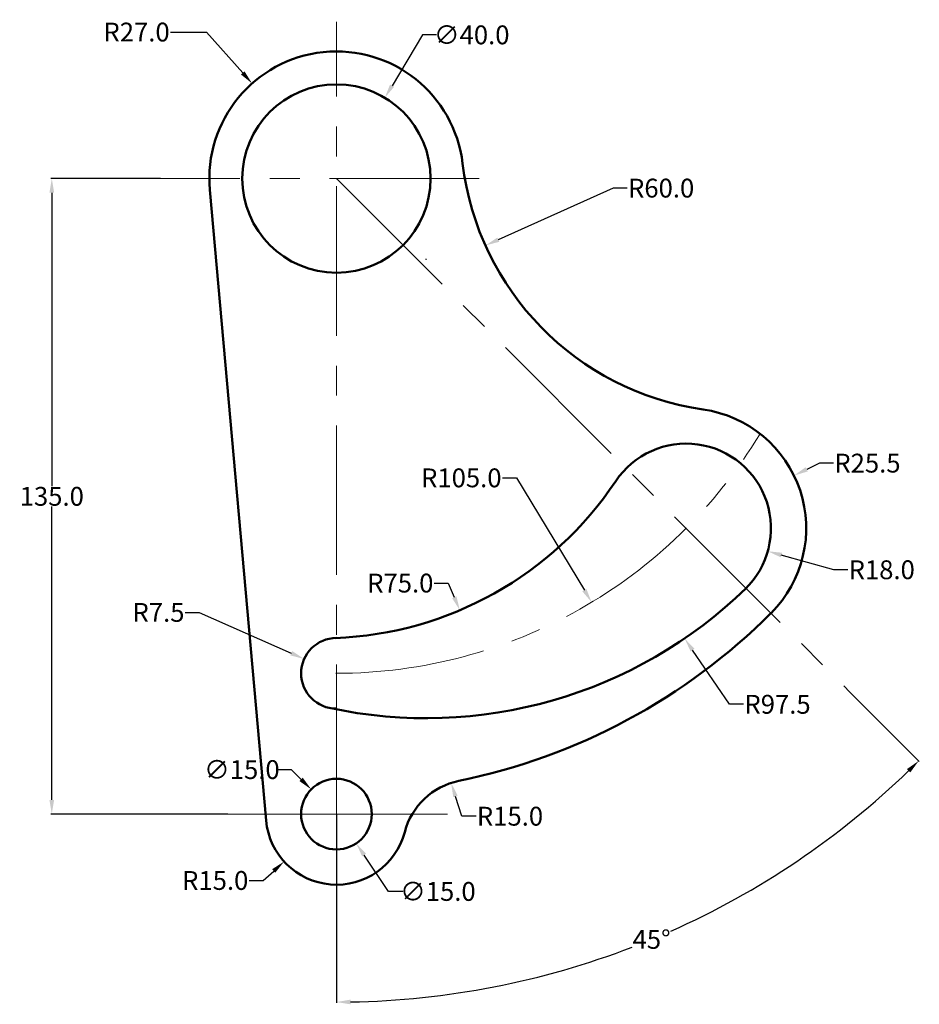
# Model space of a CAD drawing. Units: inches. Extents: x 482 to 673, y 355 to 564.
import ezdxf

# ---------------------------------------------------------------- set-up
doc = ezdxf.new("R2010")
doc.units = ezdxf.units.IN
doc.header["$MEASUREMENT"] = 0
doc.linetypes.add('CENTER', pattern=[50.8, 31.75, -6.35, 6.35, -6.35])
for name, color, linetype, lineweight in [('M-CNTR', 4, 'CENTER', 18), ('M-DIMS', 2, 'Continuous', 25), ('M-OUTL', 7, 'Continuous', 50)]:
    doc.layers.add(name, color=color, linetype=linetype, lineweight=lineweight)
doc.styles.get("Standard").update_dxf_attribs({"font": 'arial.ttf'})
doc.dimstyles.get("Standard").update_dxf_attribs({"dimtxt": 4, "dimasz": 3, "dimexe": 0.18, "dimexo": 0.0625, "dimgap": 0.09, "dimtad": 0, "dimtih": 1, "dimtoh": 1, "dimdec": 1, "dimzin": 0, "dimdsep": 46, "dimtxsty": 'Standard', "dimcen": 0.09, "dimadec": 0, "dimazin": 0, "dimtfac": 1, "dimtdec": 1, "dimtofl": 0, "dimtmove": 0, "dimatfit": 3, "dimfxl": 1, "dimtolj": 1, "dimtzin": 0, "dimarcsym": 0})

# ---------------------------------------------------------------- blocks, each defined once
blk = doc.blocks.new('*D1')
at = {"layer": 'Defpoints', "color": 0, "transparency": 16777216}
for p in [(531.06, 550.32), (548.98, 530.12)]:
    blk.add_point(p, dxfattribs=at)
at = {"layer": 'M-DIMS', "color": 0, "lineweight": -2, "transparency": 16777216}
for p, q in [((513.71, 561.24), (521.37, 561.24)), ((521.37, 561.24), (529.07, 552.56)), ((548.89, 530.12), (549.07, 530.12)), ((548.98, 530.03), (548.98, 530.21))]:
    blk.add_line(p, q, dxfattribs=at)
at = {"layer": 'M-DIMS', "color": 0, "transparency": 16777216}
blk.add_solid([(529.45, 552.89), (528.7, 552.23), (531.06, 550.32)], dxfattribs=at)
at = {"layer": 'M-DIMS', "color": 0, "transparency": 16777216, "insert": (506.52, 561.24), "char_height": 4, "attachment_point": 5}
blk.add_mtext('\\A1;R27.0', dxfattribs=at)
blk = doc.blocks.new('*D2')
at = {"layer": 'Defpoints', "color": 0, "transparency": 16777216}
for p in [(559.26, 547.28), (538.71, 512.96)]:
    blk.add_point(p, dxfattribs=at)
at = {"layer": 'M-DIMS', "color": 0, "lineweight": -2, "transparency": 16777216}
for p, q in [((567.26, 560.64), (560.8, 549.85)), ((570.26, 560.64), (567.26, 560.64)), ((548.89, 530.12), (549.07, 530.12)), ((548.98, 530.03), (548.98, 530.21))]:
    blk.add_line(p, q, dxfattribs=at)
at = {"layer": 'M-DIMS', "color": 0, "transparency": 16777216}
blk.add_solid([(560.37, 550.11), (561.23, 549.6), (559.26, 547.28)], dxfattribs=at)
at = {"layer": 'M-DIMS', "color": 0, "transparency": 16777216, "insert": (577.72, 560.64), "char_height": 4, "attachment_point": 5}
blk.add_mtext('\\A1;∅40.0', dxfattribs=at)
blk = doc.blocks.new('*D3')
at = {"layer": 'Defpoints', "color": 0, "transparency": 16777216}
for p in [(635.37, 540.47), (580.63, 515.91)]:
    blk.add_point(p, dxfattribs=at)
at = {"layer": 'M-DIMS', "color": 0, "lineweight": -2, "transparency": 16777216}
for p, q in [((607.77, 528.09), (583.36, 517.13)), ((610.77, 528.09), (607.77, 528.09))]:
    blk.add_line(p, q, dxfattribs=at)
at = {"layer": 'M-DIMS', "color": 0, "transparency": 16777216}
blk.add_solid([(583.16, 517.59), (583.57, 516.68), (580.63, 515.91)], dxfattribs=at)
at = {"layer": 'M-DIMS', "color": 0, "transparency": 16777216, "insert": (617.96, 528.09), "char_height": 4, "attachment_point": 5}
blk.add_mtext('\\A1;R60.0', dxfattribs=at)
blk = doc.blocks.new('*D4')
at = {"layer": 'Defpoints', "color": 0, "transparency": 16777216}
for p in [(646.18, 467.03), (623.28, 455.83)]:
    blk.add_point(p, dxfattribs=at)
at = {"layer": 'M-DIMS', "color": 0, "lineweight": -2, "transparency": 16777216}
for p, q in [((651.57, 469.67), (648.88, 468.35)), ((654.57, 469.67), (651.57, 469.67)), ((623.19, 455.83), (623.37, 455.83)), ((623.28, 455.74), (623.28, 455.92))]:
    blk.add_line(p, q, dxfattribs=at)
at = {"layer": 'M-DIMS', "color": 0, "transparency": 16777216}
blk.add_solid([(648.66, 468.8), (649.1, 467.9), (646.18, 467.03)], dxfattribs=at)
at = {"layer": 'M-DIMS', "color": 0, "transparency": 16777216, "insert": (661.79, 469.67), "char_height": 4, "attachment_point": 5}
blk.add_mtext('\\A1;R25.5', dxfattribs=at)
blk = doc.blocks.new('*D5')
at = {"layer": 'Defpoints', "color": 0, "transparency": 16777216}
for p in [(623.28, 455.83), (640.6, 450.96)]:
    blk.add_point(p, dxfattribs=at)
at = {"layer": 'M-DIMS', "color": 0, "lineweight": -2, "transparency": 16777216}
for p, q in [((623.19, 455.83), (623.37, 455.83)), ((623.28, 455.74), (623.28, 455.92)), ((654.63, 447.02), (643.49, 450.15)), ((657.63, 447.02), (654.63, 447.02))]:
    blk.add_line(p, q, dxfattribs=at)
at = {"layer": 'M-DIMS', "color": 0, "transparency": 16777216}
blk.add_solid([(643.63, 450.63), (643.36, 449.67), (640.6, 450.96)], dxfattribs=at)
at = {"layer": 'M-DIMS', "color": 0, "transparency": 16777216, "insert": (664.82, 447.02), "char_height": 4, "attachment_point": 5}
blk.add_mtext('\\A1;R18.0', dxfattribs=at)
blk = doc.blocks.new('*D6')
at = {"layer": 'Defpoints', "color": 0, "transparency": 16777216}
for p in [(568.03, 512.99), (622.94, 432.43)]:
    blk.add_point(p, dxfattribs=at)
at = {"layer": 'M-DIMS', "color": 0, "lineweight": -2, "transparency": 16777216}
for p, q in [((567.94, 512.99), (568.12, 512.99)), ((568.03, 512.9), (568.03, 513.08)), ((632.48, 418.44), (624.63, 429.95)), ((635.48, 418.44), (632.48, 418.44))]:
    blk.add_line(p, q, dxfattribs=at)
at = {"layer": 'M-DIMS', "color": 0, "transparency": 16777216}
blk.add_solid([(625.04, 430.23), (624.22, 429.67), (622.94, 432.43)], dxfattribs=at)
at = {"layer": 'M-DIMS', "color": 0, "transparency": 16777216, "insert": (642.69, 418.44), "char_height": 4, "attachment_point": 5}
blk.add_mtext('\\A1;R97.5', dxfattribs=at)
blk = doc.blocks.new('*D7')
at = {"layer": 'Defpoints', "color": 0, "transparency": 16777216}
for p in [(548.98, 530.03), (603.2, 440.11)]:
    blk.add_point(p, dxfattribs=at)
at = {"layer": 'M-DIMS', "color": 0, "lineweight": -2, "transparency": 16777216}
for p, q in [((584.26, 466.54), (587.26, 466.54)), ((587.26, 466.54), (601.65, 442.68))]:
    blk.add_line(p, q, dxfattribs=at)
at = {"layer": 'M-DIMS', "color": 0, "transparency": 16777216}
blk.add_solid([(602.08, 442.94), (601.22, 442.42), (603.2, 440.11)], dxfattribs=at)
at = {"layer": 'M-DIMS', "color": 0, "transparency": 16777216, "insert": (575.51, 466.54), "char_height": 4, "attachment_point": 5}
blk.add_mtext('\\A1;R105.0', dxfattribs=at)
blk = doc.blocks.new('*D8')
at = {"layer": 'Defpoints', "color": 0, "transparency": 16777216}
for p in [(545.93, 507.47), (575.19, 438.42)]:
    blk.add_point(p, dxfattribs=at)
at = {"layer": 'M-DIMS', "color": 0, "lineweight": -2, "transparency": 16777216}
for p, q in [((569.74, 444.19), (572.74, 444.19)), ((572.74, 444.19), (574.02, 441.18))]:
    blk.add_line(p, q, dxfattribs=at)
at = {"layer": 'M-DIMS', "color": 0, "transparency": 16777216}
blk.add_solid([(574.48, 441.37), (573.56, 440.98), (575.19, 438.42)], dxfattribs=at)
at = {"layer": 'M-DIMS', "color": 0, "transparency": 16777216, "insert": (562.55, 444.19), "char_height": 4, "attachment_point": 5}
blk.add_mtext('\\A1;R75.0', dxfattribs=at)
blk = doc.blocks.new('*D9')
at = {"layer": 'Defpoints', "color": 0, "transparency": 16777216}
for p in [(542.13, 428.07), (548.98, 425.03)]:
    blk.add_point(p, dxfattribs=at)
at = {"layer": 'M-DIMS', "color": 0, "lineweight": -2, "transparency": 16777216}
for p, q in [((516.84, 437.96), (519.84, 437.96)), ((519.84, 437.96), (539.39, 429.29)), ((548.89, 425.03), (549.07, 425.03)), ((548.98, 424.94), (548.98, 425.12))]:
    blk.add_line(p, q, dxfattribs=at)
at = {"layer": 'M-DIMS', "color": 0, "transparency": 16777216}
blk.add_solid([(539.59, 429.75), (539.18, 428.83), (542.13, 428.07)], dxfattribs=at)
at = {"layer": 'M-DIMS', "color": 0, "transparency": 16777216, "insert": (511.18, 437.96), "char_height": 4, "attachment_point": 5}
blk.add_mtext('\\A1;R7.5', dxfattribs=at)
blk = doc.blocks.new('*D10')
at = {"layer": 'Defpoints', "color": 0, "transparency": 16777216}
for p in [(548.98, 395.12), (537.87, 385.05)]:
    blk.add_point(p, dxfattribs=at)
at = {"layer": 'M-DIMS', "color": 0, "lineweight": -2, "transparency": 16777216}
for p, q in [((548.89, 395.12), (549.07, 395.12)), ((548.98, 395.03), (548.98, 395.21)), ((533.42, 381.02), (535.65, 383.03)), ((530.42, 381.02), (533.42, 381.02))]:
    blk.add_line(p, q, dxfattribs=at)
at = {"layer": 'M-DIMS', "color": 0, "transparency": 16777216}
blk.add_solid([(535.31, 383.4), (535.98, 382.66), (537.87, 385.05)], dxfattribs=at)
at = {"layer": 'M-DIMS', "color": 0, "transparency": 16777216, "insert": (523.23, 381.02), "char_height": 4, "attachment_point": 5}
blk.add_mtext('\\A1;R15.0', dxfattribs=at)
blk = doc.blocks.new('*D11')
at = {"layer": 'Defpoints', "color": 0, "transparency": 16777216}
for p in [(544.79, 401.34), (553.18, 388.9)]:
    blk.add_point(p, dxfattribs=at)
at = {"layer": 'M-DIMS', "color": 0, "lineweight": -2, "transparency": 16777216}
for p, q in [((548.89, 395.12), (549.07, 395.12)), ((548.98, 395.03), (548.98, 395.21)), ((560.07, 378.69), (554.86, 386.42)), ((563.07, 378.69), (560.07, 378.69))]:
    blk.add_line(p, q, dxfattribs=at)
at = {"layer": 'M-DIMS', "color": 0, "transparency": 16777216}
blk.add_solid([(555.27, 386.7), (554.44, 386.14), (553.18, 388.9)], dxfattribs=at)
at = {"layer": 'M-DIMS', "color": 0, "transparency": 16777216, "insert": (570.53, 378.69), "char_height": 4, "attachment_point": 5}
blk.add_mtext('\\A1;∅15.0', dxfattribs=at)
blk = doc.blocks.new('*D12')
at = {"layer": 'Defpoints', "color": 0, "transparency": 16777216}
for p in [(573.35, 401.74), (577.99, 387.48)]:
    blk.add_point(p, dxfattribs=at)
at = {"layer": 'M-DIMS', "color": 0, "lineweight": -2, "transparency": 16777216}
for p, q in [((575.65, 394.67), (574.28, 398.89)), ((578.65, 394.67), (575.65, 394.67))]:
    blk.add_line(p, q, dxfattribs=at)
at = {"layer": 'M-DIMS', "color": 0, "transparency": 16777216}
blk.add_solid([(574.75, 399.04), (573.8, 398.73), (573.35, 401.74)], dxfattribs=at)
at = {"layer": 'M-DIMS', "color": 0, "transparency": 16777216, "insert": (585.85, 394.67), "char_height": 4, "attachment_point": 5}
blk.add_mtext('\\A1;R15.0', dxfattribs=at)
blk = doc.blocks.new('*D13')
at = {"layer": 'Defpoints', "color": 0, "transparency": 16777216}
for p in [(548.98, 530.12), (548.98, 530.12), (657.39, 421.72), (548.98, 395.12), (594.26, 361.15)]:
    blk.add_point(p, dxfattribs=at)
at = {"layer": 'M-DIMS', "color": 0, "lineweight": -2, "transparency": 16777216}
for p, q in [((657.43, 421.67), (672.81, 406.3)), ((548.98, 395.06), (548.98, 355.01))]:
    blk.add_line(p, q, dxfattribs=at)
for start, end in [(293.9593, 314.0174), (270.9826, 291.056)]:
    blk.add_arc((548.98, 530.12), 174.93, start, end, dxfattribs=at)
at = {"layer": 'M-DIMS', "color": 0, "transparency": 16777216}
for points in [[(670.19, 404.68), (670.89, 403.97), (672.68, 406.43)], [(551.99, 354.71), (551.98, 355.71), (548.98, 355.19)]]:
    blk.add_solid(points, dxfattribs=at)
at = {"layer": 'M-DIMS', "color": 0, "transparency": 16777216, "insert": (615.93, 368.5), "char_height": 4, "attachment_point": 5}
blk.add_mtext('\\A1;45°', dxfattribs=at)
blk = doc.blocks.new('*D14')
at = {"layer": 'Defpoints', "color": 0, "transparency": 16777216}
for p in [(488.51, 530.12), (511.65, 530.12), (525.98, 395.12)]:
    blk.add_point(p, dxfattribs=at)
at = {"layer": 'M-DIMS', "color": 0, "lineweight": -2, "transparency": 16777216}
for p, q in [((511.59, 530.12), (488.33, 530.12)), ((488.51, 527.12), (488.51, 464.75)), ((488.51, 398.12), (488.51, 460.49)), ((525.92, 395.12), (488.33, 395.12))]:
    blk.add_line(p, q, dxfattribs=at)
at = {"layer": 'M-DIMS', "color": 0, "transparency": 16777216}
for points in [[(488.01, 527.12), (489.01, 527.12), (488.51, 530.12)], [(488.01, 398.12), (489.01, 398.12), (488.51, 395.12)]]:
    blk.add_solid(points, dxfattribs=at)
at = {"layer": 'M-DIMS', "color": 0, "transparency": 16777216, "insert": (488.51, 462.62), "char_height": 4, "attachment_point": 5}
blk.add_mtext('\\A1;135.0', dxfattribs=at)
blk = doc.blocks.new('*D15')
at = {"layer": 'Defpoints', "color": 0, "transparency": 16777216}
for p in [(543.63, 400.37), (554.34, 389.87)]:
    blk.add_point(p, dxfattribs=at)
at = {"layer": 'M-DIMS', "color": 0, "lineweight": -2, "transparency": 16777216}
for p, q in [((536.34, 404.57), (539.34, 404.57)), ((539.34, 404.57), (541.49, 402.47)), ((548.89, 395.12), (549.07, 395.12)), ((548.98, 395.03), (548.98, 395.21))]:
    blk.add_line(p, q, dxfattribs=at)
at = {"layer": 'M-DIMS', "color": 0, "transparency": 16777216}
blk.add_solid([(541.84, 402.83), (541.14, 402.12), (543.63, 400.37)], dxfattribs=at)
at = {"layer": 'M-DIMS', "color": 0, "transparency": 16777216, "insert": (528.89, 404.57), "char_height": 4, "attachment_point": 5}
blk.add_mtext('\\A1;∅15.0', dxfattribs=at)

msp = doc.modelspace()

# ---------------------------------------------------------------- linework, layer by layer
at = {"layer": 'M-CNTR'}
for p, q in [((548.98, 395.12), (548.98, 563.38)), ((579.29, 530.12), (511.65, 530.12)), ((548.98, 530.12), (657.39, 421.72))]:
    msp.add_line(p, q, dxfattribs=at)
msp.add_lwpolyline([(525.98, 395.12), (548.98, 395.12), (572.59, 395.12)], dxfattribs=at)
msp.add_arc((548.98, 530.03), 105, 270, 328.9838, dxfattribs=at)
at = {"layer": 'M-OUTL'}
msp.add_line((522.09, 527.72), (534.04, 393.79), dxfattribs=at)
for centre, radius in [((548.98, 530.12), 20), ((548.98, 395.12), 7.5)]:
    msp.add_circle(centre, radius, dxfattribs=at)
for centre, radius, start, end in [((548.98, 530.12), 27, 6.8321, 185.0997), ((635.37, 540.47), 60, 186.8321, 261.8702), ((623.28, 455.83), 25.5, 315, 81.8702), ((623.28, 455.83), 18, 314.0246, 146.2672), ((545.93, 507.47), 75, 272.1194, 326.2672), ((568.03, 512.99), 97.5, 257.7856, 314.2046), ((548.98, 530.12), 130.56, 281.4957, 315), ((548.98, 425.03), 7.5, 90, 270), ((577.99, 387.48), 15, 101.4957, 165.2391), ((548.98, 395.12), 15, 185.0997, 345.2391)]:
    msp.add_arc(centre, radius, start, end, dxfattribs=at)

# ---------------------------------------------------------------- dimensions: what is measured, and where the dimension line sits
at = {"layer": 'M-DIMS'}
for center, mpoint, picture, middle in [((548.98, 530.12), (531.06, 550.32), '*D1', (506.52, 561.24)), ((635.37, 540.47), (580.63, 515.91), '*D3', (617.96, 528.09)), ((548.98, 530.03), (603.2, 440.11), '*D7', (575.51, 466.54)), ((568.03, 512.99), (622.94, 432.43), '*D6', (642.69, 418.44)), ((545.93, 507.47), (575.19, 438.42), '*D8', (562.55, 444.19)), ((623.28, 455.83), (640.6, 450.96), '*D5', (664.82, 447.02)), ((548.98, 425.03), (542.13, 428.07), '*D9', (511.18, 437.96)), ((577.99, 387.48), (573.35, 401.74), '*D12', (585.85, 394.67))]:
    dim = msp.add_radius_dim(center=center, mpoint=mpoint, dimstyle='Standard', override={"dimclrd": 0, "dimclre": 0, "dimclrt": 0}, dxfattribs=at)
    dim.commit()
    dim.dimension.update_dxf_attribs({"geometry": picture, "text_midpoint": middle, "dimtype": 164})
for p1, p2, override, picture, middle in [((538.71, 512.96), (559.26, 547.28), {"dimclrd": 0, "dimclre": 0, "dimclrt": 0}, '*D2', (577.72, 560.64)), ((554.34, 389.87), (543.63, 400.37), {"dimdec": 1, "dimlfac": 1, "dimrnd": 0, "dimzin": 0, "dimdsep": 46, "dimlunit": 2}, '*D15', (528.89, 404.57)), ((544.79, 401.34), (553.18, 388.9), {"dimclrd": 0, "dimclre": 0, "dimclrt": 0}, '*D11', (570.53, 378.69))]:
    dim = msp.add_diameter_dim_2p(p1=p1, p2=p2, dimstyle='Standard', override=override, dxfattribs=at)
    dim.commit()
    dim.dimension.update_dxf_attribs({"geometry": picture, "text_midpoint": middle, "dimtype": 163})
dim = msp.add_linear_dim(base=(488.51, 530.12), p1=(525.98, 395.12), p2=(511.65, 530.12), angle=90, dimstyle='Standard', override={"dimclrd": 0, "dimclre": 0, "dimclrt": 0}, dxfattribs=at)
dim.commit()
dim.dimension.update_dxf_attribs({"geometry": '*D14', "text_midpoint": (488.51, 462.62)})
dim = msp.add_angular_dim_2l(base=(594.26, 361.15), line1=((548.98, 530.12), (657.39, 421.72)), line2=((548.98, 530.12), (548.98, 395.12)), dimstyle='Standard', override={"dimclrd": 0, "dimclre": 0, "dimclrt": 0}, dxfattribs=at)
dim.commit()
dim.dimension.update_dxf_attribs({"geometry": '*D13', "text_midpoint": (615.93, 368.5)})
for center, mpoint, picture, middle in [((623.28, 455.83), (646.18, 467.03), '*D4', (661.79, 469.67)), ((548.98, 395.12), (537.87, 385.05), '*D10', (523.23, 381.02))]:
    dim = msp.add_radius_dim(center=center, mpoint=mpoint, dimstyle='Standard', override={"dimclrd": 0, "dimclre": 0, "dimclrt": 0}, dxfattribs=at)
    dim.commit()
    dim.dimension.update_dxf_attribs({"geometry": picture, "text_midpoint": middle})

doc.saveas('drawing.dxf')
